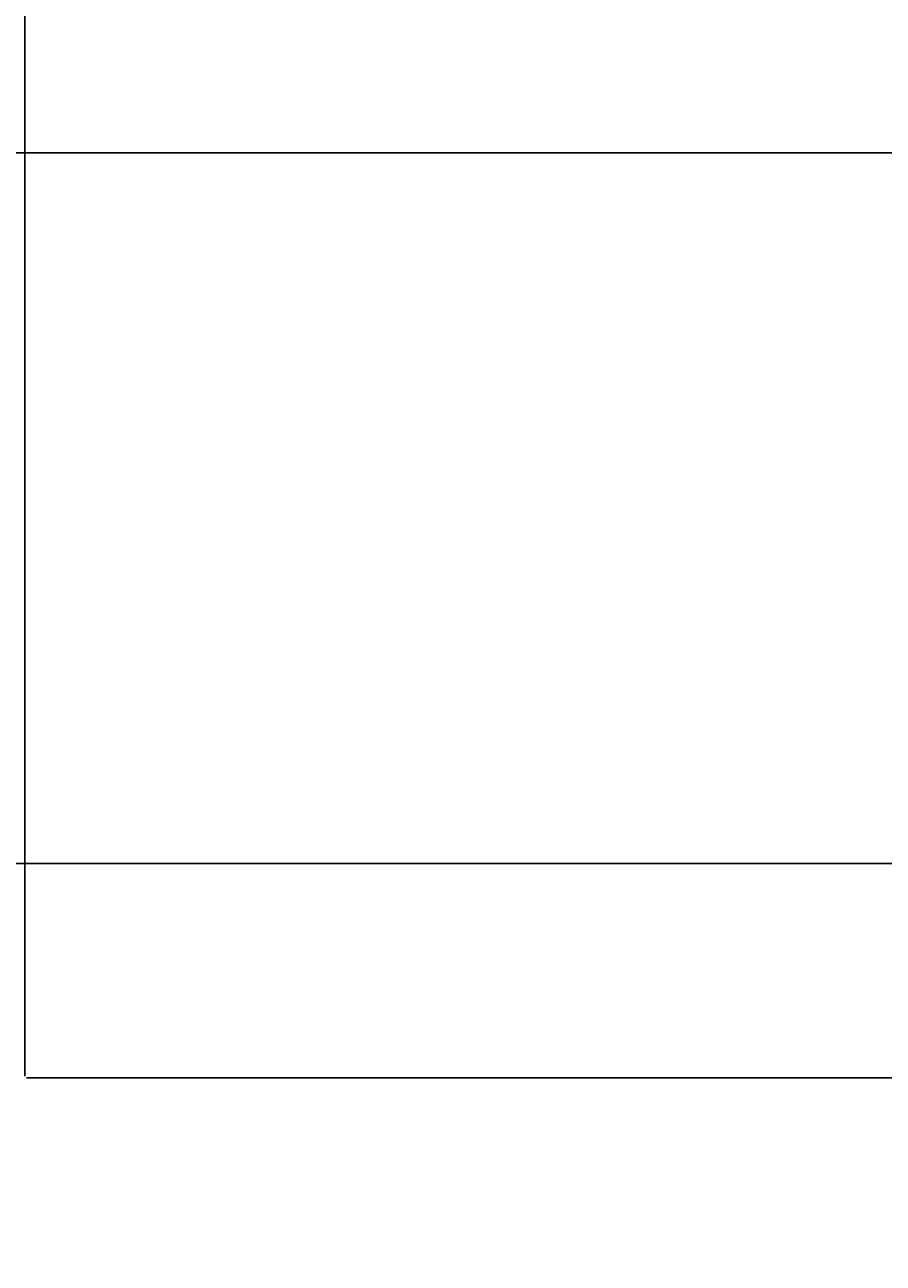
# Model space of a CAD drawing. Units: inches. Extents: x 1998 to 2588, y 1139 to 1977.
# Tile 14 of 134: x 2115 to 2147, y 1622 to 1668. Entities that reach past the tile are written whole.
import ezdxf

# ---------------------------------------------------------------- set-up
doc = ezdxf.new("R2010")
doc.units = ezdxf.units.IN
doc.layers.add('A-ANNO-DIMS', color=2, linetype='Continuous', lineweight=18)
doc.styles.get("Standard").update_dxf_attribs({"font": 'arial.ttf'})
doc.dimstyles.get("Standard").update_dxf_attribs({"dimtxt": 0.18, "dimasz": 0.18, "dimexe": 0.18, "dimexo": 0.0625, "dimgap": 0.09, "dimtad": 0, "dimtih": 1, "dimtoh": 1, "dimdec": 4, "dimzin": 0, "dimdsep": 46, "dimtxsty": 'Standard', "dimcen": 0.09, "dimadec": 0, "dimazin": 0, "dimtfac": 1, "dimtdec": 4, "dimtofl": 0, "dimtmove": 0, "dimatfit": 3, "dimfxl": 1, "dimtolj": 1, "dimtzin": 0, "dimarcsym": 0})

# ---------------------------------------------------------------- blocks, each defined once
blk = doc.blocks.new('*D30')
at = {"layer": 'A-ANNO-DIMS', "color": 0, "lineweight": -2, "transparency": 16777216}
for p, q in [((2407.91, 1636.732), (1997.843, 1636.732)), ((1998.023, 1636.552), (1998.023, 1615.913)), ((1998.023, 1594.912), (1998.023, 1615.552)), ((2407.91, 1594.732), (1997.843, 1594.732))]:
    blk.add_line(p, q, dxfattribs=at)
at = {"layer": 'A-ANNO-DIMS', "color": 0, "transparency": 16777216}
for points in [[(1997.993, 1636.552), (1998.053, 1636.552), (1998.023, 1636.732)], [(1997.993, 1594.912), (1998.053, 1594.912), (1998.023, 1594.732)]]:
    blk.add_solid(points, dxfattribs=at)
at = {"layer": 'Defpoints', "color": 0, "transparency": 16777216}
for p in [(1998.023, 1636.732), (2407.973, 1636.732), (2407.973, 1594.732)]:
    blk.add_point(p, dxfattribs=at)
at = {"layer": 'A-ANNO-DIMS', "color": 0, "transparency": 16777216, "insert": (1998.023, 1615.732), "char_height": 0.18, "attachment_point": 5}
blk.add_mtext('\\A1;42', dxfattribs=at)
blk = doc.blocks.new('*D38')
at = {"layer": 'A-ANNO-DIMS', "color": 0, "lineweight": -2, "transparency": 16777216}
for p, q in [((2197.387, 1663.247), (1997.843, 1663.247)), ((1998.023, 1663.067), (1998.023, 1638.171)), ((1998.023, 1612.912), (1998.023, 1637.808)), ((2197.387, 1612.732), (1997.843, 1612.732))]:
    blk.add_line(p, q, dxfattribs=at)
at = {"layer": 'A-ANNO-DIMS', "color": 0, "transparency": 16777216}
for points in [[(1997.993, 1663.067), (1998.053, 1663.067), (1998.023, 1663.247)], [(1997.993, 1612.912), (1998.053, 1612.912), (1998.023, 1612.732)]]:
    blk.add_solid(points, dxfattribs=at)
at = {"layer": 'Defpoints', "color": 0, "transparency": 16777216}
for p in [(1998.023, 1663.247), (2197.45, 1663.247), (2197.45, 1612.732)]:
    blk.add_point(p, dxfattribs=at)
at = {"layer": 'A-ANNO-DIMS', "color": 0, "transparency": 16777216, "insert": (1998.023, 1637.99), "char_height": 0.18, "attachment_point": 5}
blk.add_mtext('\\A1;50.51', dxfattribs=at)
blk = doc.blocks.new('*D39')
at = {"layer": 'A-ANNO-DIMS', "color": 0, "lineweight": -2, "transparency": 16777216}
for p, q in [((2115.035, 1628.742), (2588.309, 1628.742)), ((2588.129, 1628.562), (2588.129, 1612.685)), ((2588.129, 1596.444), (2588.129, 1612.321)), ((2115.035, 1596.264), (2588.309, 1596.264))]:
    blk.add_line(p, q, dxfattribs=at)
at = {"layer": 'A-ANNO-DIMS', "color": 0, "transparency": 16777216}
for points in [[(2588.099, 1628.562), (2588.159, 1628.562), (2588.129, 1628.742)], [(2588.099, 1596.444), (2588.159, 1596.444), (2588.129, 1596.264)]]:
    blk.add_solid(points, dxfattribs=at)
at = {"layer": 'Defpoints', "color": 0, "transparency": 16777216}
for p in [(2114.973, 1628.742), (2588.129, 1628.742), (2114.973, 1596.264)]:
    blk.add_point(p, dxfattribs=at)
at = {"layer": 'A-ANNO-DIMS', "color": 0, "transparency": 16777216, "insert": (2588.129, 1612.503), "char_height": 0.18, "attachment_point": 5}
blk.add_mtext('\\A1;32.48', dxfattribs=at)
blk = doc.blocks.new('*D40')
at = {"layer": 'A-ANNO-DIMS', "color": 0, "lineweight": -2, "transparency": 16777216}
for p, q in [((2105.973, 1628.541), (2105.973, 1977.362)), ((2106.153, 1977.182), (2110.324, 1977.182)), ((2114.793, 1977.182), (2110.622, 1977.182)), ((2114.973, 1628.804), (2114.973, 1977.362))]:
    blk.add_line(p, q, dxfattribs=at)
at = {"layer": 'A-ANNO-DIMS', "color": 0, "transparency": 16777216}
for points in [[(2106.153, 1977.212), (2106.153, 1977.152), (2105.973, 1977.182)], [(2114.793, 1977.212), (2114.793, 1977.152), (2114.973, 1977.182)]]:
    blk.add_solid(points, dxfattribs=at)
at = {"layer": 'Defpoints', "color": 0, "transparency": 16777216}
for p in [(2114.973, 1977.182), (2114.973, 1628.742), (2105.973, 1628.478)]:
    blk.add_point(p, dxfattribs=at)
at = {"layer": 'A-ANNO-DIMS', "color": 0, "transparency": 16777216, "insert": (2110.473, 1977.182), "char_height": 0.18, "attachment_point": 5}
blk.add_mtext('\\A1;9', dxfattribs=at)

msp = doc.modelspace()

# ---------------------------------------------------------------- dimensions: what is measured, and where the dimension line sits
at = {"layer": 'A-ANNO-DIMS'}
dim = msp.add_linear_dim(base=(2114.9729, 1977.1824), p1=(2105.9729, 1628.4781), p2=(2114.9729, 1628.7416), dimstyle='Standard', override={"dimdec": 0, "dimlfac": 1, "dimrnd": 0, "dimzin": 0, "dimdsep": 46, "dimlunit": 2}, dxfattribs=at)
dim.commit()
dim.dimension.update_dxf_attribs({"geometry": '*D40', "text_midpoint": (2110.4729, 1977.1824)})
for base, p1, p2, override, picture, middle in [((1998.0229, 1663.2466), (2197.4499, 1612.7324), (2197.4499, 1663.2466), {"dimdec": 2, "dimlfac": 1, "dimrnd": 0, "dimzin": 0, "dimdsep": 46, "dimlunit": 2}, '*D38', (1998.0229, 1637.9895)), ((1998.0229, 1636.7324), (2407.9729, 1594.7324), (2407.9729, 1636.7324), {"dimdec": 0, "dimlfac": 1, "dimrnd": 0, "dimzin": 0, "dimdsep": 46, "dimlunit": 2}, '*D30', (1998.0229, 1615.7324)), ((2588.1286, 1628.7416), (2114.9729, 1596.2642), (2114.9729, 1628.7416), {"dimdec": 2, "dimlfac": 1, "dimrnd": 0, "dimzin": 0, "dimdsep": 46, "dimlunit": 2}, '*D39', (2588.1286, 1612.5029))]:
    dim = msp.add_linear_dim(base=base, p1=p1, p2=p2, angle=90, dimstyle='Standard', override=override, dxfattribs=at)
    dim.commit()
    dim.dimension.update_dxf_attribs({"geometry": picture, "text_midpoint": middle})

doc.saveas('drawing.dxf')
